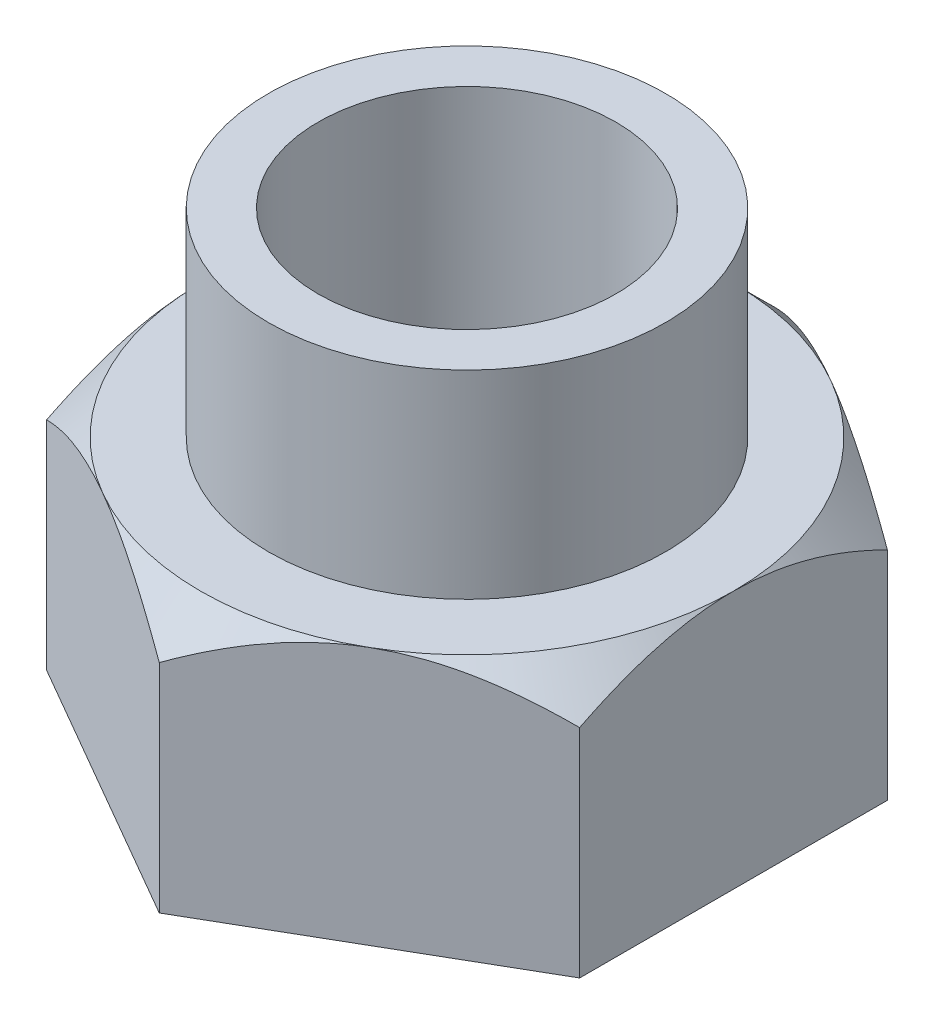
from build123d import *

# Parameters (mm, degrees)
HEX_BODY_DEPTH                  = 65
CORNER_CHAMFER_SKETCH_OUTSIDE_W = 309.254
CORNER_CHAMFER_SKETCH_OUTSIDE_H = 330.02
CORNER_CHAMFER_SKETCH_OUTSIDE_R = 67.116968793
HEX_CORNER_CHAMFER_45DEG_DEPTH  = 65
HEX_CORNER_CHAMFER_45DEG_DRAFT  = -45
LOCKING_COLLAR_SKETCH_R         = 50
LOCKING_COLLAR_SKETCH_R_2       = 37.5
LOCKING_COLLAR_DEPTH            = 50
NUT_START                       = -120
SKETCH3_2_R                     = 37.5
NUT_BORE_DEPTH                  = 120


with BuildPart() as part:
    # Hex Profile Sketch → Hex Body (new body)
    with BuildSketch(Plane(origin=(0, 0, 0), x_dir=(1, 0, 0), z_dir=(0, 1, 0))):
        Polygon((0, -77.5), (67.116968793, -38.75), (67.116968793, 38.75), (0, 77.5), (-67.116968793, 38.75), (-67.116968793, -38.75), align=None)
    extrude(amount=HEX_BODY_DEPTH)


with BuildPart() as hex_corner_chamfer_45deg_tool:
    # Corner Chamfer Sketch outside → Hex Corner Chamfer 45deg (with draft: the straight prism first)
    with BuildSketch(Plane(origin=(0, 65, 0), x_dir=(1, 0, 0), z_dir=(0, 1, 0))):
        Rectangle(CORNER_CHAMFER_SKETCH_OUTSIDE_W, CORNER_CHAMFER_SKETCH_OUTSIDE_H)
        Circle(CORNER_CHAMFER_SKETCH_OUTSIDE_R, mode=Mode.SUBTRACT)
    extrude(amount=-HEX_CORNER_CHAMFER_45DEG_DEPTH)
    # Hex Corner Chamfer 45deg: the draft: its side faces are tilted about the plane it starts from
    hex_corner_chamfer_45deg_sides = [hex_corner_chamfer_45deg_tool.faces().sort_by_distance(p)[0] for p in [
        (0, 32.5, 165.01),
        (154.627, 32.5, 0),
        (0, 32.5, -165.01),
        (-154.627, 32.5, 0),
        (-67.116968793, 32.5, 0),
    ]]
    draft(hex_corner_chamfer_45deg_sides, Plane(origin=(0, 65, 0), x_dir=(1, 0, 0), z_dir=(0, 1, 0)), HEX_CORNER_CHAMFER_45DEG_DRAFT)


with BuildPart() as part_1:
    add(part.part)

    # Hex Corner Chamfer 45deg: cut by hex_corner_chamfer_45deg_tool
    add(hex_corner_chamfer_45deg_tool.part, mode=Mode.SUBTRACT)

    # Locking Collar Sketch → Locking Collar (add)
    with BuildSketch(Plane(origin=(0, 65, 0), x_dir=(1, 0, 0), z_dir=(0, 1, 0))):
        with Locations(Location((0, 0, 0), (0, 0, 270))):
            Circle(LOCKING_COLLAR_SKETCH_R)
        with Locations(Location((0, 0, 0), (0, 0, 270))):
            Circle(LOCKING_COLLAR_SKETCH_R_2, mode=Mode.SUBTRACT)
    extrude(amount=LOCKING_COLLAR_DEPTH)

    # Sketch3_2 → Nut Bore (cut)
    with BuildSketch(Plane(origin=(0, 65, 0), x_dir=(1, 0, 0), z_dir=(0, 1, 0)).offset(NUT_START)):
        with Locations(Location((0, 0, 0), (0, 0, 270))):
            Circle(SKETCH3_2_R)
    extrude(amount=NUT_BORE_DEPTH, mode=Mode.SUBTRACT)


solid = part_1.part
